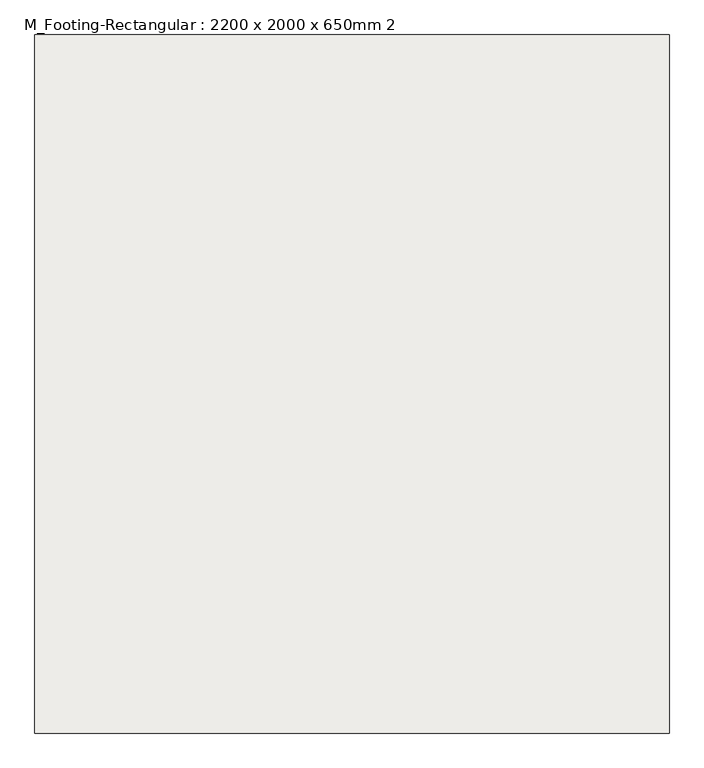
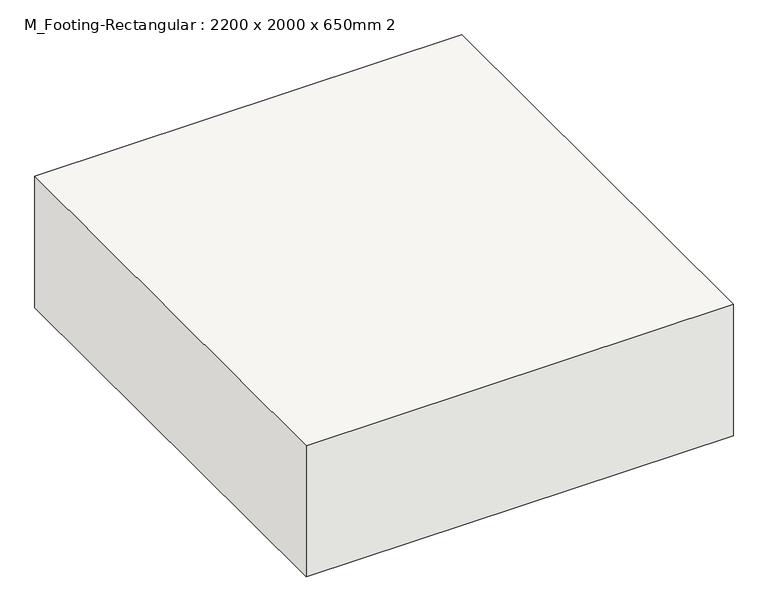
"""IFC4 building model written with IfcOpenShell, lengths in millimetres: slab geometry, M_Footing-Rectangular : 2200 x 2000 x 650mm 2."""

from ifc_helpers import new_model, si_unit, frame, origin, place, context, project, spatial, polyline, outline, extrude, source, transform, mapped, element, save


def m_footing_rectangular_2200_x_2000_x_650mm_2_4a7b59ae(model_context):
    return source(origin(), model_context, "Body", "SweptSolid", [
        extrude(outline(polyline([(1000.0, 1100.0), (1000.0, -1100.0), (-1000.0, -1100.0), (-1000.0, 1100.0), (1000.0, 1100.0)])), frame((0.0, 0.0, -650.0), z_axis=(0.0, 0.0, 1.0), x_axis=(1.0, 0.0, 0.0)), (0.0, 0.0, 1.0), 650.0),
    ])


if __name__ == "__main__":
    model = new_model("IFC4")
    model_context = context("Model", 3, world=origin())
    ifc_project = project(units=[si_unit("LENGTHUNIT", "METRE", prefix="MILLI")], contexts=[model_context])
    site = spatial("IfcSite", under=ifc_project)
    building = spatial("IfcBuilding", under=site)
    placement = place(None, origin())
    m_footing_rectangular_2200_x_2000_x_650mm_2_shape = m_footing_rectangular_2200_x_2000_x_650mm_2_4a7b59ae(model_context)
    element("IfcSlab", 1, ObjectType="M_Footing-Rectangular : 2200 x 2000 x 650mm 2", at=placement, inside=building, context=model_context, shape_type="MappedRepresentation", body=[
        mapped(m_footing_rectangular_2200_x_2000_x_650mm_2_shape, transform((0.0, 0.0, 0.0), x_axis=(1.0, 0.0, 0.0), y_axis=(0.0, 1.0, 0.0), z_axis=(0.0, 0.0, 1.0))),
    ])
    save(model, "model.ifc")

# Revit data of these elements
# Type "M_Footing-Rectangular : 2200 x 2000 x 650mm 2"
#   Width = 2000 mm
#   Length = 2200 mm
#   Foundation Thickness = 650 mm
#   Structural Material [instance default] = Concrete, Cast-in-Place gray
#   Assembly Code = ""
# Element 1 (IfcSlab, "M_Footing-Rectangular : 2200 x 2000 x 650mm 2")
#   Materials on its faces: "Concrete, Cast-in-Place gray"
# Materials
#   "Concrete, Cast-in-Place gray": class "Concrete", colour RGB 192 192 192, transparency 0, Description = "Cast-in-place concrete", Cost = 0
